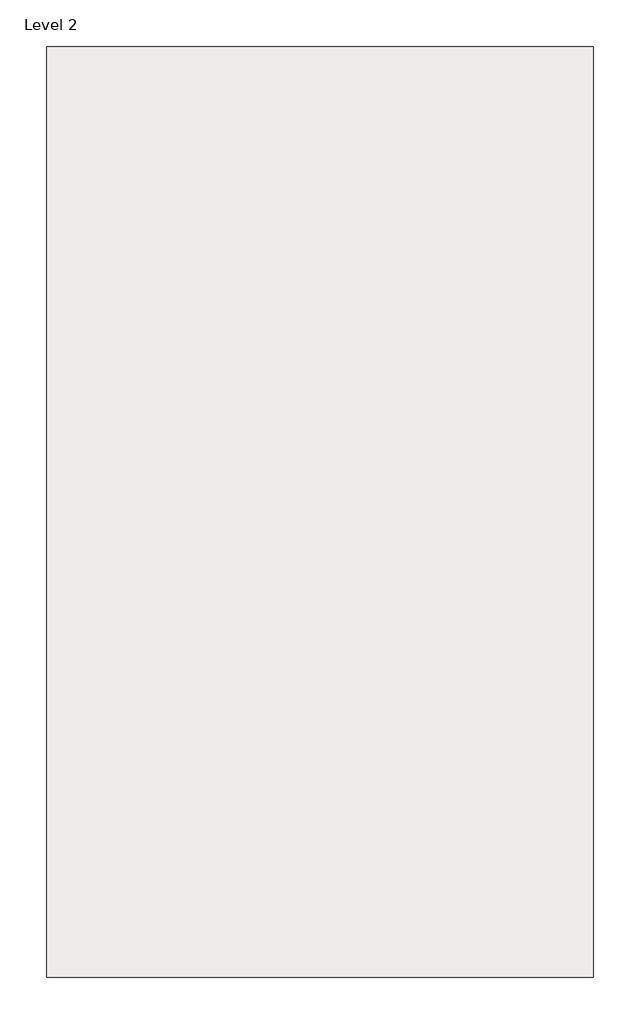
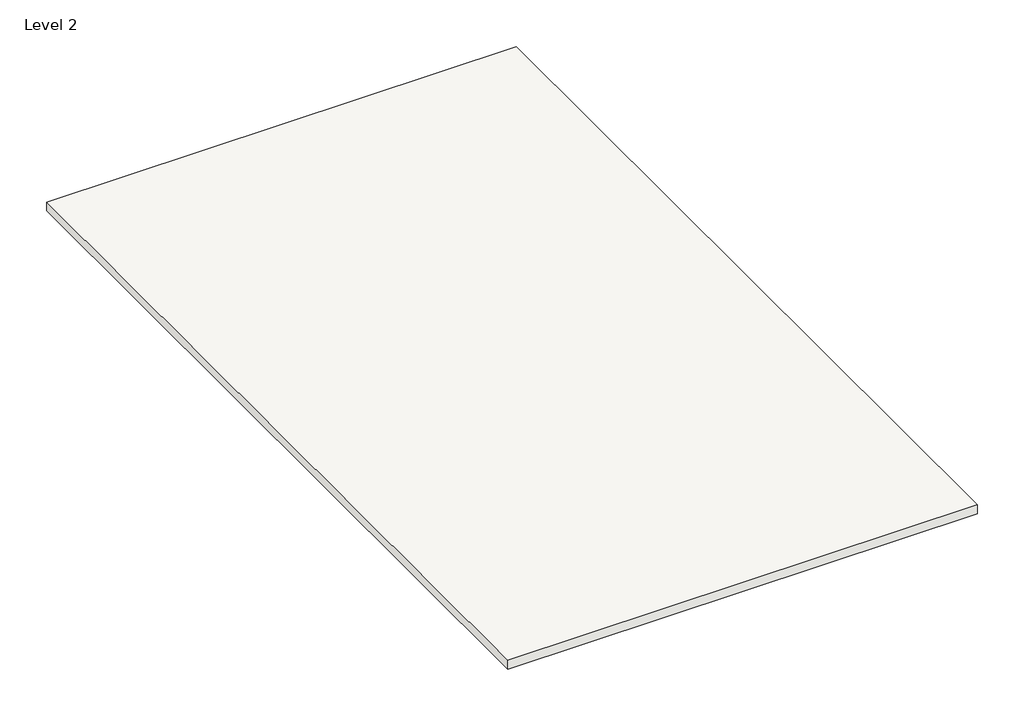
# One storey, incomplete: 1 roof.
"""IFC4 building model written with IfcOpenShell, lengths in millimetres."""

from ifc_helpers import new_model, si_unit, frame, origin, place, context, project, spatial, polyline, outline, extrude, element, save

model = new_model("IFC4")

# Units and contexts
model_context = context("Model", 3, world=origin())
ifc_project = project(units=[si_unit("LENGTHUNIT", "METRE", prefix="MILLI")], contexts=[model_context])

# Site, building, storey
site = spatial("IfcSite", under=ifc_project)
building = spatial("IfcBuilding", under=site)
storey = spatial("IfcBuildingStorey", under=building, Name="Level 2", Elevation=3048.0)

# Roof
placement = place(None, origin())
element("IfcRoof", 1, ObjectType="Generic - 12\"", at=placement, inside=storey, context=model_context, shape_type="SweptSolid", body=[
    extrude(outline(polyline([(-5222.940747, 7243.7935985), (2587.559253, 7243.7935985), (2587.559253, -6053.1064015), (-5222.940747, -6053.1064015), (-5222.940747, 7243.7935985)])), frame((0.0, 0.0, 3048.0), z_axis=(0.0, 0.0, 1.0), x_axis=(1.0, 0.0, 0.0)), (0.0, 0.0, 1.0), 152.4),
])

save(model, "model.ifc")

# Revit data of these elements
# Type "Generic - 12\""
#   Assembly Code = "B1020"
#   Layers, outside or top first: 0' - 6" no material (function 1)
# Element 1 (IfcRoof, "Generic - 12\"")
#   built-in parameter 1001705 = 10.5 (stored number, unit not read)
#   built-in parameter 1001710 = 33615
#   Phase Created = New Construction
#   Materials on its faces: "Default Roof"
# Materials
#   "Default Roof": colour RGB 88 101 114, transparency 0, Cost = 0
